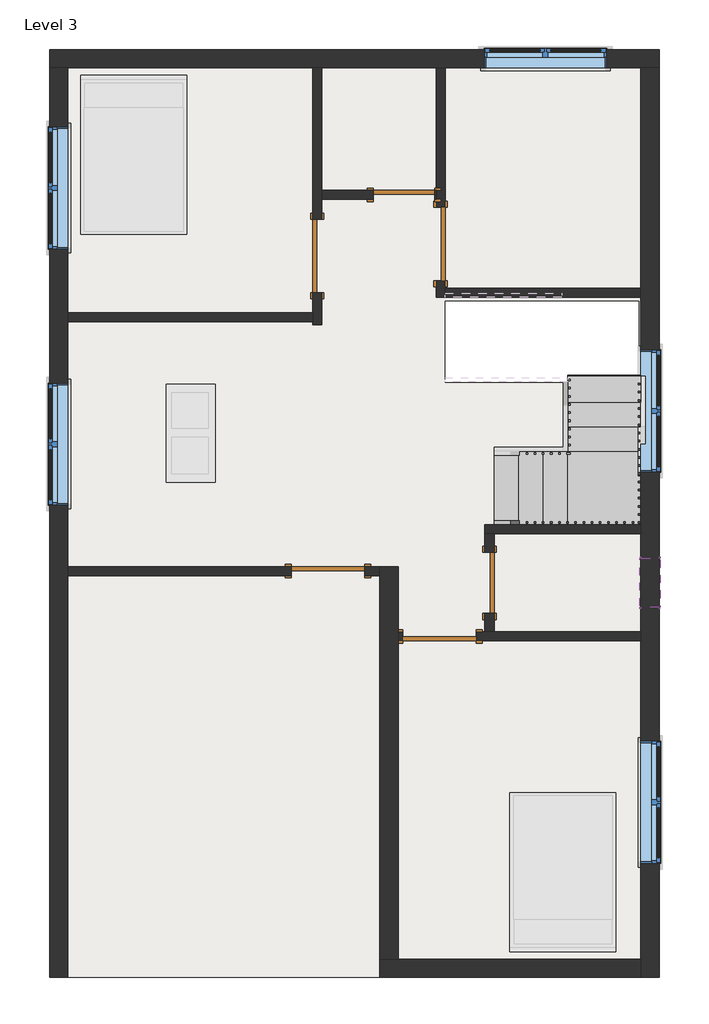
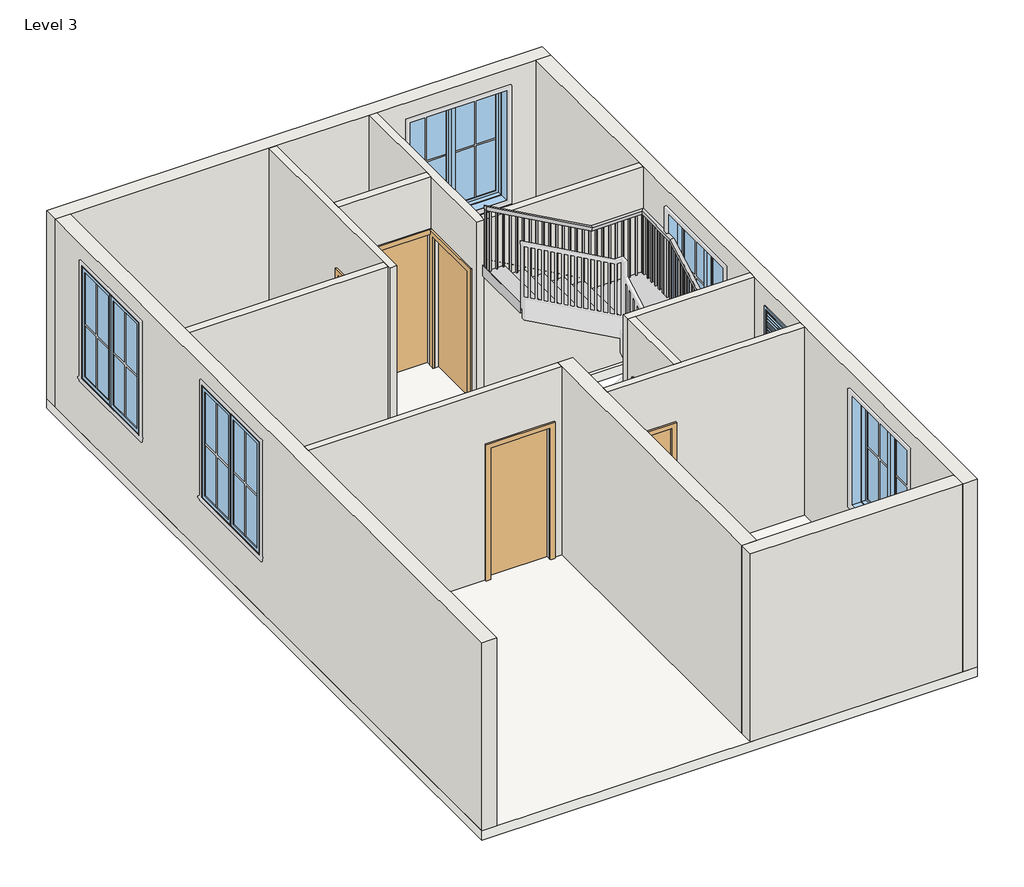
# One storey, part 1 of 2: 14 walls, 6 doors, 6 windows, 1 railing, 1 slab, 1 stair flight.
# Revit data of these elements (continued)
# Element 28 (IfcWindow, "Window-Casement-Double : WIN 5'") (continued)
#   Exterior Wall Closure = 0' - 1 1/4"
#   Interior Trim Visibility = yes
#   Exterior Trim Visibility = yes
#   Phase Created = New Construction
#   Materials on its faces: "Wood - Stained", "Glass", "Clad - White"
# Element 29 (IfcWindow, "Window-Louvers : 24\" x 24\"")
#   Mark = "12"
#   Blade Width = 1' - 10 1/2"
#   Phase Created = New Construction
#   Materials on its faces: "Birch"
# Materials
#   "Door - Panel": class "Wood", colour RGB 210 159 95, transparency 0, Cost = 0
#   "Door - Frame": colour RGB 118 70 51, transparency 0, Cost = 0
#   "Wood - Stained": class "Wood", colour RGB 224 178 126, transparency 0, Cost = 0
#   "Glass": class "Glass", colour RGB 0 128 192, transparency 0.75, Description = "Soda Lime Glass", Cost = 0
#   "Clad - White": class "Wood", colour RGB 242 242 238, transparency 0, Cost = 0
#   "Birch": class "Wood", colour RGB 224 178 126, transparency 0, Description = "Betula Alleghaniensis", Cost = 0
#   "Default Floor": colour RGB 128 128 128, transparency 0, Cost = 0
#   "Default Wall": colour RGB 128 128 128, transparency 0, Cost = 0
#   "Copper": class "Metal", colour RGB 0 0 0, transparency 0, Description = "Copper, matte finish", Cost = 0
